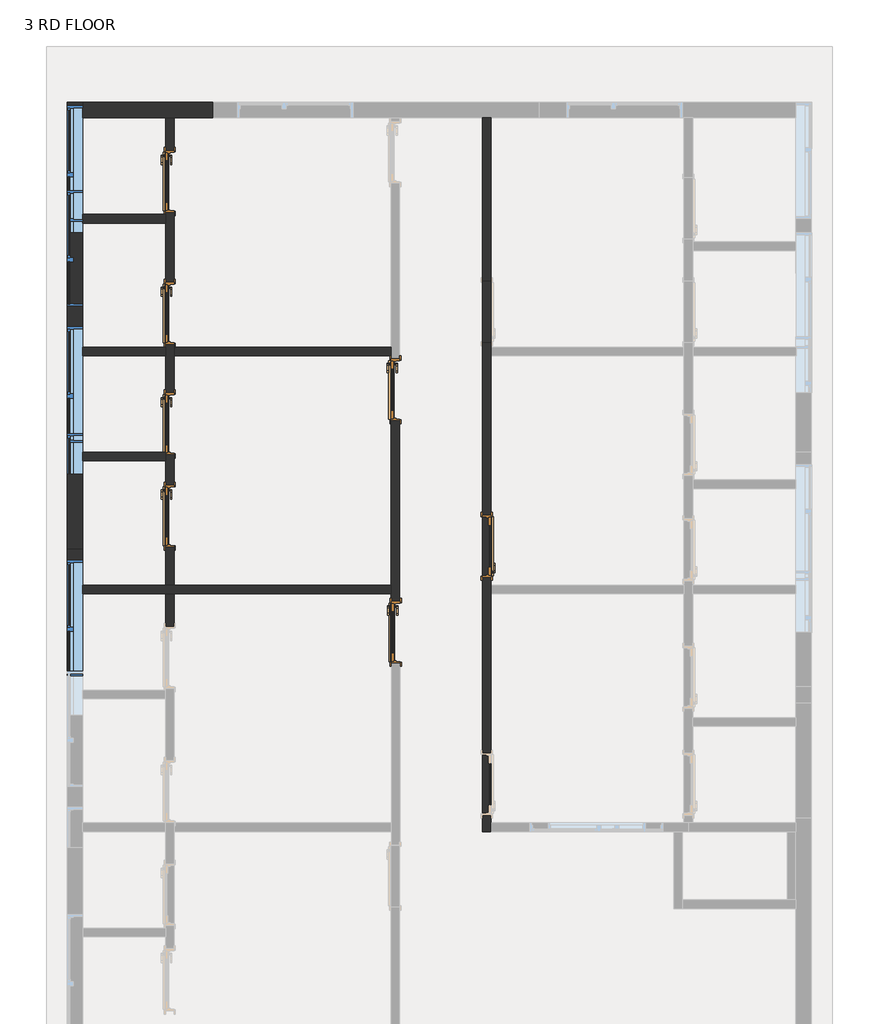
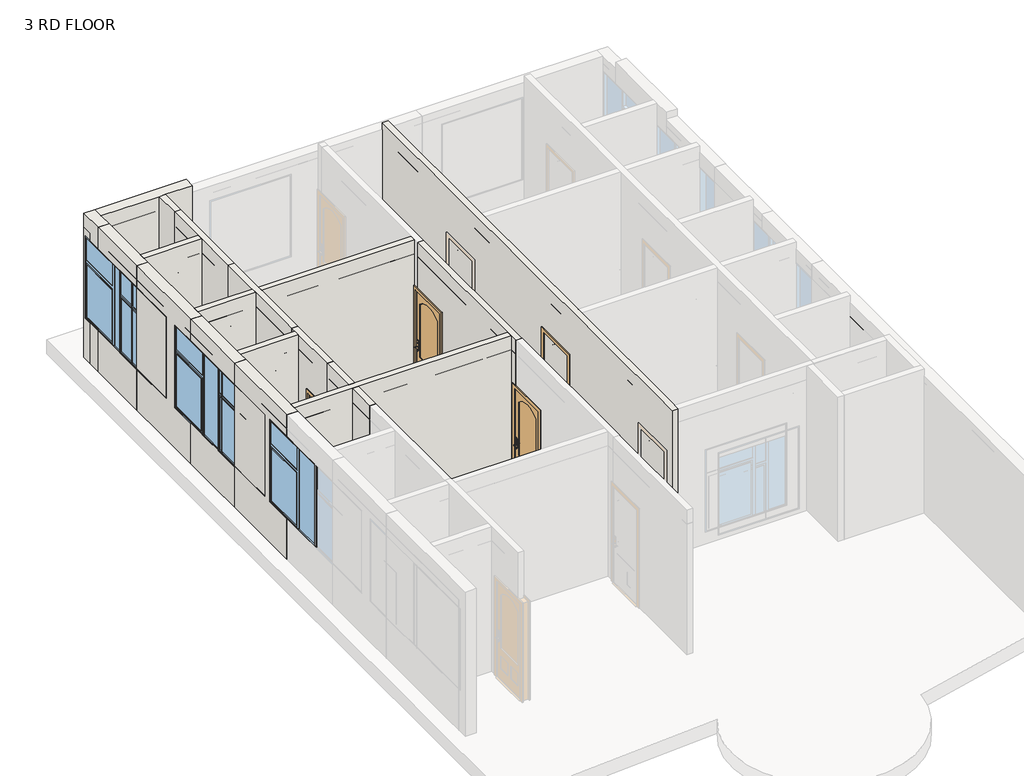
# One storey, part 2 of 5: 35 walls, 7 doors, 6 windows.
"""IFC4 building model written with IfcOpenShell, lengths in millimetres."""

from ifc_helpers import new_model, si_unit, frame, origin, place, context, project, spatial, polyline, outline, extrude, faceted_brep, transform, mapped, element, save
from components import door_346b4a94, m_window_casement_double_sidelight_1702_x_1829mm_c8b42c7f

model = new_model("IFC4")

# Units and contexts
model_context = context("Model", 3, world=origin())
ifc_project = project(units=[si_unit("LENGTHUNIT", "METRE", prefix="MILLI")], contexts=[model_context])

# Site, building, storey
site = spatial("IfcSite", under=ifc_project)
building = spatial("IfcBuilding", under=site)
storey = spatial("IfcBuildingStorey", under=building, Name="3 RD FLOOR", Elevation=9601.2)

# Doors
placement = place(None, origin())
door_shape = door_346b4a94(model_context)
element("IfcDoor", 1, ObjectType="2'10\"X7'", at=placement, inside=storey, context=model_context, shape_type="MappedRepresentation", body=[
    mapped(door_shape, transform((-273.0358866, 1471.0399728, 9601.2), x_axis=(0.0, -1.0, 0.0), y_axis=(1.0, 0.0, 0.0), z_axis=(0.0, 0.0, 1.0))),
])
element("IfcDoor", 2, ObjectType="2'10\"X7'", at=placement, inside=storey, context=model_context, shape_type="MappedRepresentation", body=[
    mapped(door_shape, transform((-4952.9858866, 3273.6174518, 9601.2), x_axis=(0.0, 1.0, 0.0), y_axis=(-1.0, 0.0, 0.0), z_axis=(0.0, 0.0, 1.0))),
])
element("IfcDoor", 3, ObjectType="2'10\"X7'", at=placement, inside=storey, context=model_context, shape_type="MappedRepresentation", body=[
    mapped(door_shape, transform((-4952.9858866, 4900.320652, 9601.2), x_axis=(0.0, 1.0, 0.0), y_axis=(-1.0, 0.0, 0.0), z_axis=(0.0, 0.0, 1.0))),
])
element("IfcDoor", 4, ObjectType="2'10\"X7'", at=placement, inside=storey, context=model_context, shape_type="MappedRepresentation", body=[
    mapped(door_shape, transform((-4952.9858866, 6843.9929737, 9601.2), x_axis=(0.0, 1.0, 0.0), y_axis=(-1.0, 0.0, 0.0), z_axis=(0.0, 0.0, 1.0))),
])
element("IfcDoor", 5, ObjectType="2'10\"X7'", at=placement, inside=storey, context=model_context, shape_type="MappedRepresentation", body=[
    mapped(door_shape, transform((-1625.1621817, 3775.8008884, 9601.2), x_axis=(0.0, 1.0, 0.0), y_axis=(-1.0, 0.0, 0.0), z_axis=(0.0, 0.0, 1.0))),
])
element("IfcDoor", 6, ObjectType="2'10\"X7'", at=placement, inside=storey, context=model_context, shape_type="MappedRepresentation", body=[
    mapped(door_shape, transform((-1620.1577262, 202.9637706, 9601.2), x_axis=(0.0, 1.0, 0.0), y_axis=(-1.0, 0.0, 0.0), z_axis=(0.0, 0.0, 1.0))),
])
element("IfcDoor", 7, ObjectType="2'10\"X7'", at=placement, inside=storey, context=model_context, shape_type="MappedRepresentation", body=[
    mapped(door_shape, transform((-4952.9858866, 1913.3521609, 9601.2), x_axis=(0.0, 1.0, 0.0), y_axis=(-1.0, 0.0, 0.0), z_axis=(0.0, 0.0, 1.0))),
])

# Walls
element("IfcWall", 8, ObjectType="Generic - 4.5\"", at=placement, inside=storey, context=model_context, shape_type="Brep", body=[
    faceted_brep([(-5013.3108866, 7224.9929737, 12801.6), (-5013.3108866, 7782.9399728, 12801.6), (-5013.3108866, 7782.9399728, 9601.2), (-5013.3108866, 7300.7929737, 9601.2), (-5013.3108866, 7300.7929737, 11759.8), (-5013.3108866, 7224.9929737, 11759.8), (-5013.3108866, 7224.9929737, 12496.8), (-4886.3108866, 7782.9399728, 12801.6), (-4886.3108866, 7224.9929737, 12801.6), (-4886.3108866, 7224.9929737, 12496.8), (-4886.3108866, 7224.9929737, 11759.8), (-4886.3108866, 7300.7929737, 11759.8), (-4886.3108866, 7300.7929737, 9601.2), (-4886.3108866, 7782.9399728, 9601.2)], [[[0, 1, 2, 3, 4, 5, 6]], [[7, 8, 9, 10, 11, 12, 13]], [[2, 13, 12, 3]], [[1, 0, 8, 7]], [[11, 4, 3, 12]], [[4, 11, 10, 5]], [[8, 0, 6, 5, 10, 9]], [[1, 7, 13, 2]]]),
])
element("IfcWall", 9, ObjectType="Generic - 4.5\"", at=placement, inside=storey, context=model_context, shape_type="Brep", body=[
    faceted_brep([(-5013.3108866, 5281.320652, 12801.6), (-5013.3108866, 6233.5399728, 12801.6), (-5013.3108866, 6360.5399728, 12801.6), (-5013.3108866, 7224.9929737, 12801.6), (-5013.3108866, 7224.9929737, 12496.8), (-5013.3108866, 7224.9929737, 11759.8), (-5013.3108866, 6387.1929737, 11759.8), (-5013.3108866, 6387.1929737, 9601.2), (-5013.3108866, 6360.5399728, 9601.2), (-5013.3108866, 6233.5399728, 9601.2), (-5013.3108866, 5357.120652, 9601.2), (-5013.3108866, 5357.120652, 11759.8), (-5013.3108866, 5281.320652, 11759.8), (-5013.3108866, 5281.320652, 12496.8), (-4886.3108866, 7224.9929737, 12801.6), (-4886.3108866, 5281.320652, 12801.6), (-4886.3108866, 5281.320652, 12496.8), (-4886.3108866, 5281.320652, 11759.8), (-4886.3108866, 5357.120652, 11759.8), (-4886.3108866, 5357.120652, 9601.2), (-4886.3108866, 6387.1929737, 9601.2), (-4886.3108866, 6387.1929737, 11759.8), (-4886.3108866, 7224.9929737, 11759.8), (-4886.3108866, 7224.9929737, 12496.8)], [[[0, 1, 2, 3, 4, 5, 6, 7, 8, 9, 10, 11, 12, 13]], [[14, 15, 16, 17, 18, 19, 20, 21, 22, 23]], [[19, 10, 9, 8, 7, 20]], [[3, 2, 1, 0, 15, 14]], [[18, 11, 10, 19]], [[11, 18, 17, 12]], [[21, 6, 5, 22]], [[6, 21, 20, 7]], [[15, 0, 13, 12, 17, 16]], [[3, 14, 23, 22, 5, 4]]]),
])
element("IfcWall", 10, ObjectType="Generic - 4.5\"", at=placement, inside=storey, context=model_context, shape_type="SweptSolid", body=[
    extrude(outline(polyline([(-5013.3108866, 6233.5399728), (-6232.5508078, 6233.5399728), (-6232.5508078, 6360.5399728), (-5013.3108866, 6360.5399728), (-5013.3108866, 6233.5399728)])), frame((0.0, 0.0, 9601.2), z_axis=(0.0, 0.0, 1.0), x_axis=(1.0, 0.0, 0.0)), (0.0, 0.0, 1.0), 3200.4),
])
element("IfcWall", 11, ObjectType="Generic - 4.5\"", at=placement, inside=storey, context=model_context, shape_type="SweptSolid", body=[
    extrude(outline(polyline([(-5013.3108866, 4277.7399728), (-6232.5508078, 4277.7399728), (-6232.5508078, 4404.7399728), (-5013.3108866, 4404.7399728), (-5013.3108866, 4277.7399728)])), frame((0.0, 0.0, 9601.2), z_axis=(0.0, 0.0, 1.0), x_axis=(1.0, 0.0, 0.0)), (0.0, 0.0, 1.0), 3200.4),
])
element("IfcWall", 12, ObjectType="Generic - 4.5\"", at=placement, inside=storey, context=model_context, shape_type="Brep", body=[
    faceted_brep([(-5013.3108866, 2968.8174518, 12801.6), (-5013.3108866, 4277.7399728, 12801.6), (-5013.3108866, 4404.7399728, 12801.6), (-5013.3108866, 5281.320652, 12801.6), (-5013.3108866, 5281.320652, 12496.8), (-5013.3108866, 5281.320652, 11759.8), (-5013.3108866, 4443.520652, 11759.8), (-5013.3108866, 4443.520652, 9601.2), (-5013.3108866, 4404.7399728, 9601.2), (-5013.3108866, 4277.7399728, 9601.2), (-5013.3108866, 3730.4174518, 9601.2), (-5013.3108866, 3730.4174518, 11759.8), (-5013.3108866, 2968.8174518, 11759.8), (-5013.3108866, 2968.8174518, 12496.8), (-4886.3108866, 5281.320652, 12801.6), (-4886.3108866, 4404.7399728, 12801.6), (-4886.3108866, 4277.7399728, 12801.6), (-4886.3108866, 2968.8174518, 12801.6), (-4886.3108866, 2968.8174518, 12496.8), (-4886.3108866, 2968.8174518, 11759.8), (-4886.3108866, 3730.4174518, 11759.8), (-4886.3108866, 3730.4174518, 9601.2), (-4886.3108866, 4277.7399728, 9601.2), (-4886.3108866, 4404.7399728, 9601.2), (-4886.3108866, 4443.520652, 9601.2), (-4886.3108866, 4443.520652, 11759.8), (-4886.3108866, 5281.320652, 11759.8), (-4886.3108866, 5281.320652, 12496.8)], [[[0, 1, 2, 3, 4, 5, 6, 7, 8, 9, 10, 11, 12, 13]], [[14, 15, 16, 17, 18, 19, 20, 21, 22, 23, 24, 25, 26, 27]], [[21, 10, 9, 8, 7, 24, 23, 22]], [[3, 2, 1, 0, 17, 16, 15, 14]], [[20, 11, 10, 21]], [[11, 20, 19, 12]], [[25, 6, 5, 26]], [[6, 25, 24, 7]], [[3, 14, 27, 26, 5, 4]], [[17, 0, 13, 12, 19, 18]]]),
])
element("IfcWall", 13, ObjectType="Generic - 4.5\"", at=placement, inside=storey, context=model_context, shape_type="Brep", body=[
    faceted_brep([(-6232.5508078, 2728.3399728, 9601.2), (-5013.3108866, 2728.3399728, 9601.2), (-5013.3108866, 2728.3399728, 12801.6), (-6232.5508078, 2728.3399728, 12801.6), (-6232.5508078, 2855.3399728, 9601.2), (-6232.5508078, 2855.3399728, 12801.6), (-5013.3108866, 2855.3399728, 12801.6), (-5013.3108866, 2855.3399728, 9601.2), (-5013.3108866, 2816.8174518, 9601.2)], [[[0, 1, 2, 3]], [[4, 5, 6, 7]], [[1, 0, 4, 7, 8]], [[3, 2, 6, 5]], [[0, 3, 5, 4]], [[2, 1, 8, 7, 6]]]),
])
element("IfcWall", 14, ObjectType="Generic - 4.5\"", at=placement, inside=storey, context=model_context, shape_type="Brep", body=[
    faceted_brep([(-5013.3108866, 1684.7521609, 12801.6), (-5013.3108866, 2728.3399728, 12801.6), (-5013.3108866, 2855.3399728, 12801.6), (-5013.3108866, 2968.8174518, 12801.6), (-5013.3108866, 2968.8174518, 12496.8), (-5013.3108866, 2968.8174518, 11759.8), (-5013.3108866, 2816.8174518, 11759.8), (-5013.3108866, 2816.8174518, 9601.2), (-5013.3108866, 2728.3399728, 9601.2), (-5013.3108866, 2370.1521609, 9601.2), (-5013.3108866, 2370.1521609, 11759.8), (-5013.3108866, 1684.7521609, 11759.8), (-5013.3108866, 1684.7521609, 12496.8), (-4886.3108866, 2968.8174518, 12801.6), (-4886.3108866, 1684.7521609, 12801.6), (-4886.3108866, 1684.7521609, 12496.8), (-4886.3108866, 1684.7521609, 11759.8), (-4886.3108866, 2370.1521609, 11759.8), (-4886.3108866, 2370.1521609, 9601.2), (-4886.3108866, 2816.8174518, 9601.2), (-4886.3108866, 2816.8174518, 11759.8), (-4886.3108866, 2968.8174518, 11759.8), (-4886.3108866, 2968.8174518, 12496.8)], [[[0, 1, 2, 3, 4, 5, 6, 7, 8, 9, 10, 11, 12]], [[13, 14, 15, 16, 17, 18, 19, 20, 21, 22]], [[7, 19, 18, 9, 8]], [[3, 2, 1, 0, 14, 13]], [[20, 6, 5, 21]], [[6, 20, 19, 7]], [[17, 10, 9, 18]], [[10, 17, 16, 11]], [[3, 13, 22, 21, 5, 4]], [[14, 0, 12, 11, 16, 15]]]),
])
element("IfcWall", 15, ObjectType="Generic - 4.5\"", at=placement, inside=storey, context=model_context, shape_type="Brep", body=[
    faceted_brep([(-6232.5508078, 772.5399728, 9601.2), (-5013.3108866, 772.5399728, 9601.2), (-4886.3108866, 772.5399728, 9601.2), (-1685.9108866, 772.5399728, 9601.2), (-1685.9108866, 772.5399728, 12801.6), (-4886.3108866, 772.5399728, 12801.6), (-5013.3108866, 772.5399728, 12801.6), (-6232.5508078, 772.5399728, 12801.6), (-6232.5508078, 899.5399728, 9601.2), (-6232.5508078, 899.5399728, 12801.6), (-5013.3108866, 899.5399728, 12801.6), (-4886.3108866, 899.5399728, 12801.6), (-1685.9108866, 899.5399728, 12801.6), (-1685.9108866, 899.5399728, 9601.2), (-4886.3108866, 899.5399728, 9601.2), (-5013.3108866, 899.5399728, 9601.2)], [[[0, 1, 2, 3, 4, 5, 6, 7]], [[8, 9, 10, 11, 12, 13, 14, 15]], [[3, 2, 1, 0, 8, 15, 14, 13]], [[4, 3, 13, 12]], [[7, 6, 5, 4, 12, 11, 10, 9]], [[0, 7, 9, 8]]]),
])
element("IfcWall", 16, ObjectType="Generic - 4.5\"", at=placement, inside=storey, context=model_context, shape_type="Brep", body=[
    faceted_brep([(-5013.3108866, 288.8295043, 9601.2), (-5013.3108866, 288.8295043, 11759.8), (-5013.3108866, 136.8295043, 11759.8), (-5013.3108866, 136.8295043, 12496.8), (-5013.3108866, 136.8295043, 12801.6), (-5013.3108866, 772.5399728, 12801.6), (-5013.3108866, 772.5399728, 9601.2), (-4886.3108866, 288.8295043, 11759.8), (-4886.3108866, 288.8295043, 9601.2), (-4886.3108866, 772.5399728, 9601.2), (-4886.3108866, 772.5399728, 12801.6), (-4886.3108866, 136.8295043, 12801.6), (-4886.3108866, 136.8295043, 12496.8), (-4886.3108866, 136.8295043, 11759.8)], [[[0, 1, 2, 3, 4, 5, 6]], [[7, 8, 9, 10, 11, 12, 13]], [[8, 0, 6, 9]], [[4, 11, 10, 5]], [[7, 1, 0, 8]], [[1, 7, 13, 2]], [[6, 5, 10, 9]], [[11, 4, 3, 2, 13, 12]]]),
    faceted_brep([(-5013.3108866, 1684.7521609, 11759.8), (-5013.3108866, 1456.5521609, 11759.8), (-5013.3108866, 1456.5521609, 9601.2), (-5013.3108866, 899.5399728, 9601.2), (-5013.3108866, 899.5399728, 12801.6), (-5013.3108866, 1684.7521609, 12801.6), (-5013.3108866, 1684.7521609, 12496.8), (-4886.3108866, 1456.5521609, 11759.8), (-4886.3108866, 1684.7521609, 11759.8), (-4886.3108866, 1684.7521609, 12496.8), (-4886.3108866, 1684.7521609, 12801.6), (-4886.3108866, 899.5399728, 12801.6), (-4886.3108866, 899.5399728, 9601.2), (-4886.3108866, 1456.5521609, 9601.2)], [[[0, 1, 2, 3, 4, 5, 6]], [[7, 8, 9, 10, 11, 12, 13]], [[2, 13, 12, 3]], [[10, 5, 4, 11]], [[4, 3, 12, 11]], [[7, 1, 0, 8]], [[1, 7, 13, 2]], [[5, 10, 9, 8, 0, 6]]]),
])
element("IfcWall", 17, ObjectType="Generic - 4.5\"", at=placement, inside=storey, context=model_context, shape_type="SweptSolid", body=[
    extrude(outline(polyline([(-1685.9108866, 4277.7399728), (-4886.3108866, 4277.7399728), (-4886.3108866, 4404.7399728), (-1685.9108866, 4404.7399728), (-1685.9108866, 4277.7399728)])), frame((0.0, 0.0, 9601.2), z_axis=(0.0, 0.0, 1.0), x_axis=(1.0, 0.0, 0.0)), (0.0, 0.0, 1.0), 3200.4),
])
element("IfcWall", 18, ObjectType="Generic - 4.5\"", at=placement, inside=storey, context=model_context, shape_type="Brep", body=[
    faceted_brep([(-1685.4871817, 609.3637706, 12801.6), (-1685.4871817, 4182.2008884, 12801.6), (-1685.4871817, 4182.2008884, 11759.8), (-1685.4871817, 3319.0008884, 11759.8), (-1685.4871817, 3319.0008884, 9601.2), (-1685.4871817, 659.7637706, 9601.2), (-1685.4871817, 659.7637706, 11759.8), (-1685.4871817, 609.3637706, 11759.8), (-1558.4871817, 4182.2008884, 12801.6), (-1558.4871817, 609.3637706, 12801.6), (-1558.4871817, 609.3637706, 11759.8), (-1558.4871817, 659.7637706, 11759.8), (-1558.4871817, 659.7637706, 9601.2), (-1558.4871817, 3319.0008884, 9601.2), (-1558.4871817, 3319.0008884, 11759.8), (-1558.4871817, 4182.2008884, 11759.8), (-1680.4827262, 609.3637706, 12801.6), (-1558.9108866, 4182.2008884, 12801.6), (-1558.9108866, 4182.2008884, 11759.8), (-1680.4827262, 609.3637706, 11759.8)], [[[0, 1, 2, 3, 4, 5, 6, 7]], [[8, 9, 10, 11, 12, 13, 14, 15]], [[4, 13, 12, 5]], [[1, 0, 16, 9, 8, 17]], [[14, 3, 2, 18, 15]], [[3, 14, 13, 4]], [[11, 6, 5, 12]], [[6, 11, 10, 19, 7]], [[9, 16, 0, 7, 19, 10]], [[1, 17, 8, 15, 18, 2]]]),
])
element("IfcWall", 19, ObjectType="Generic - 4.5\"", at=placement, inside=storey, context=model_context, shape_type="Brep", body=[
    faceted_brep([(-339.7108866, -2732.6600272, 12801.6), (-339.7108866, 7782.9399728, 12801.6), (-339.7108866, 7782.9399728, 9601.2), (-339.7108866, 5382.2399728, 9601.2), (-339.7108866, 5382.2399728, 11759.8), (-339.7108866, 4468.6399728, 11759.8), (-339.7108866, 4468.6399728, 9601.2), (-339.7108866, 1927.8399728, 9601.2), (-339.7108866, 1927.8399728, 11759.8), (-339.7108866, 1014.2399728, 11759.8), (-339.7108866, 1014.2399728, 9601.2), (-339.7108866, -1577.3600272, 9601.2), (-339.7108866, -1577.3600272, 11759.8), (-339.7108866, -2490.9600272, 11759.8), (-339.7108866, -2490.9600272, 9601.2), (-339.7108866, -2732.6600272, 9601.2), (-212.7108866, 7782.9399728, 12801.6), (-212.7108866, 4404.7399728, 12801.6), (-212.7108866, 4277.7399728, 12801.6), (-212.7108866, 899.5399728, 12801.6), (-212.7108866, 772.5399728, 12801.6), (-212.7108866, -2605.6600272, 12801.6), (-212.7108866, -2732.6600272, 12801.6), (-212.7108866, -2732.6600272, 12496.8), (-212.7108866, -2732.6600272, 9601.2), (-212.7108866, -2605.6600272, 9601.2), (-212.7108866, -2490.9600272, 9601.2), (-212.7108866, -2490.9600272, 11759.8), (-212.7108866, -1577.3600272, 11759.8), (-212.7108866, -1577.3600272, 9601.2), (-212.7108866, 772.5399728, 9601.2), (-212.7108866, 899.5399728, 9601.2), (-212.7108866, 1014.2399728, 9601.2), (-212.7108866, 1014.2399728, 11759.8), (-212.7108866, 1927.8399728, 11759.8), (-212.7108866, 1927.8399728, 9601.2), (-212.7108866, 4277.7399728, 9601.2), (-212.7108866, 4404.7399728, 9601.2), (-212.7108866, 4468.6399728, 9601.2), (-212.7108866, 4468.6399728, 11759.8), (-212.7108866, 5382.2399728, 11759.8), (-212.7108866, 5382.2399728, 9601.2), (-212.7108866, 7782.9399728, 9601.2)], [[[0, 1, 2, 3, 4, 5, 6, 7, 8, 9, 10, 11, 12, 13, 14, 15]], [[16, 17, 18, 19, 20, 21, 22, 23, 24, 25, 26, 27, 28, 29, 30, 31, 32, 33, 34, 35, 36, 37, 38, 39, 40, 41, 42]], [[24, 15, 14, 26, 25]], [[29, 11, 10, 32, 31, 30]], [[35, 7, 6, 38, 37, 36]], [[2, 42, 41, 3]], [[1, 0, 22, 21, 20, 19, 18, 17, 16]], [[13, 27, 26, 14]], [[27, 13, 12, 28]], [[28, 12, 11, 29]], [[9, 33, 32, 10]], [[33, 9, 8, 34]], [[34, 8, 7, 35]], [[5, 39, 38, 6]], [[39, 5, 4, 40]], [[40, 4, 3, 41]], [[15, 24, 23, 22, 0]], [[1, 16, 42, 2]]]),
])
element("IfcWall", 20, ObjectType="Generic - 4.5\"", at=placement, inside=storey, context=model_context, shape_type="SweptSolid", body=[
    extrude(outline(polyline([(7782.9399728, 12496.8), (7782.9399728, 9601.2), (7300.7929737, 9601.2), (7300.7929737, 11759.8), (7224.9929737, 11759.8), (7224.9929737, 12496.8), (7782.9399728, 12496.8)])), frame((-5013.3108866, 0.0, 0.0), z_axis=(1.0, 0.0, 0.0), x_axis=(0.0, 1.0, 0.0)), (0.0, 0.0, 1.0), 127.0),
])
element("IfcWall", 21, ObjectType="Generic - 4.5\"", at=placement, inside=storey, context=model_context, shape_type="Brep", body=[
    faceted_brep([(-5013.3108866, 5281.320652, 12496.8), (-5013.3108866, 6233.5399728, 12496.8), (-5013.3108866, 6360.5399728, 12496.8), (-5013.3108866, 7224.9929737, 12496.8), (-5013.3108866, 7224.9929737, 11759.8), (-5013.3108866, 6387.1929737, 11759.8), (-5013.3108866, 6387.1929737, 9601.2), (-5013.3108866, 6360.5399728, 9601.2), (-5013.3108866, 6233.5399728, 9601.2), (-5013.3108866, 5357.120652, 9601.2), (-5013.3108866, 5357.120652, 11759.8), (-5013.3108866, 5281.320652, 11759.8), (-4886.3108866, 7224.9929737, 12496.8), (-4886.3108866, 5281.320652, 12496.8), (-4886.3108866, 5281.320652, 11759.8), (-4886.3108866, 5357.120652, 11759.8), (-4886.3108866, 5357.120652, 9601.2), (-4886.3108866, 6387.1929737, 9601.2), (-4886.3108866, 6387.1929737, 11759.8), (-4886.3108866, 7224.9929737, 11759.8)], [[[0, 1, 2, 3, 4, 5, 6, 7, 8, 9, 10, 11]], [[12, 13, 14, 15, 16, 17, 18, 19]], [[16, 9, 8, 7, 6, 17]], [[13, 0, 11, 14]], [[3, 12, 19, 4]], [[3, 2, 1, 0, 13, 12]], [[18, 5, 4, 19]], [[5, 18, 17, 6]], [[15, 10, 9, 16]], [[10, 15, 14, 11]]]),
])
element("IfcWall", 22, ObjectType="Generic - 4.5\"", at=placement, inside=storey, context=model_context, shape_type="SweptSolid", body=[
    extrude(outline(polyline([(-5013.3108866, 6233.5399728), (-6232.5508078, 6233.5399728), (-6232.5508078, 6360.5399728), (-5013.3108866, 6360.5399728), (-5013.3108866, 6233.5399728)])), frame((0.0, 0.0, 9601.2), z_axis=(0.0, 0.0, 1.0), x_axis=(1.0, 0.0, 0.0)), (0.0, 0.0, 1.0), 2895.6),
])
element("IfcWall", 23, ObjectType="Generic - 4.5\"", at=placement, inside=storey, context=model_context, shape_type="SweptSolid", body=[
    extrude(outline(polyline([(-5013.3108866, 4277.7399728), (-6232.5508078, 4277.7399728), (-6232.5508078, 4404.7399728), (-5013.3108866, 4404.7399728), (-5013.3108866, 4277.7399728)])), frame((0.0, 0.0, 9601.2), z_axis=(0.0, 0.0, 1.0), x_axis=(1.0, 0.0, 0.0)), (0.0, 0.0, 1.0), 2895.6),
])
element("IfcWall", 24, ObjectType="Generic - 4.5\"", at=placement, inside=storey, context=model_context, shape_type="Brep", body=[
    faceted_brep([(-5013.3108866, 2968.8174518, 12496.8), (-5013.3108866, 4277.7399728, 12496.8), (-5013.3108866, 4404.7399728, 12496.8), (-5013.3108866, 5281.320652, 12496.8), (-5013.3108866, 5281.320652, 11759.8), (-5013.3108866, 4443.520652, 11759.8), (-5013.3108866, 4443.520652, 9601.2), (-5013.3108866, 4404.7399728, 9601.2), (-5013.3108866, 4277.7399728, 9601.2), (-5013.3108866, 3730.4174518, 9601.2), (-5013.3108866, 3730.4174518, 11759.8), (-5013.3108866, 2968.8174518, 11759.8), (-4886.3108866, 5281.320652, 12496.8), (-4886.3108866, 4404.7399728, 12496.8), (-4886.3108866, 4277.7399728, 12496.8), (-4886.3108866, 2968.8174518, 12496.8), (-4886.3108866, 2968.8174518, 11759.8), (-4886.3108866, 3730.4174518, 11759.8), (-4886.3108866, 3730.4174518, 9601.2), (-4886.3108866, 4277.7399728, 9601.2), (-4886.3108866, 4404.7399728, 9601.2), (-4886.3108866, 4443.520652, 9601.2), (-4886.3108866, 4443.520652, 11759.8), (-4886.3108866, 5281.320652, 11759.8)], [[[0, 1, 2, 3, 4, 5, 6, 7, 8, 9, 10, 11]], [[12, 13, 14, 15, 16, 17, 18, 19, 20, 21, 22, 23]], [[18, 9, 8, 7, 6, 21, 20, 19]], [[15, 0, 11, 16]], [[3, 12, 23, 4]], [[3, 2, 1, 0, 15, 14, 13, 12]], [[22, 5, 4, 23]], [[5, 22, 21, 6]], [[17, 10, 9, 18]], [[10, 17, 16, 11]]]),
])
element("IfcWall", 25, ObjectType="Generic - 4.5\"", at=placement, inside=storey, context=model_context, shape_type="Brep", body=[
    faceted_brep([(-6232.5508078, 2728.3399728, 9601.2), (-5013.3108866, 2728.3399728, 9601.2), (-5013.3108866, 2728.3399728, 12496.8), (-6232.5508078, 2728.3399728, 12496.8), (-6232.5508078, 2855.3399728, 9601.2), (-6232.5508078, 2855.3399728, 12496.8), (-5013.3108866, 2855.3399728, 12496.8), (-5013.3108866, 2855.3399728, 9601.2), (-5013.3108866, 2816.8174518, 9601.2)], [[[0, 1, 2, 3]], [[4, 5, 6, 7]], [[1, 0, 4, 7, 8]], [[0, 3, 5, 4]], [[2, 1, 8, 7, 6]], [[3, 2, 6, 5]]]),
])
element("IfcWall", 26, ObjectType="Generic - 4.5\"", at=placement, inside=storey, context=model_context, shape_type="Brep", body=[
    faceted_brep([(-5013.3108866, 1684.7521609, 12496.8), (-5013.3108866, 2728.3399728, 12496.8), (-5013.3108866, 2855.3399728, 12496.8), (-5013.3108866, 2968.8174518, 12496.8), (-5013.3108866, 2968.8174518, 11759.8), (-5013.3108866, 2816.8174518, 11759.8), (-5013.3108866, 2816.8174518, 9601.2), (-5013.3108866, 2728.3399728, 9601.2), (-5013.3108866, 2370.1521609, 9601.2), (-5013.3108866, 2370.1521609, 11759.8), (-5013.3108866, 1684.7521609, 11759.8), (-4886.3108866, 2968.8174518, 12496.8), (-4886.3108866, 1684.7521609, 12496.8), (-4886.3108866, 1684.7521609, 11759.8), (-4886.3108866, 2370.1521609, 11759.8), (-4886.3108866, 2370.1521609, 9601.2), (-4886.3108866, 2816.8174518, 9601.2), (-4886.3108866, 2816.8174518, 11759.8), (-4886.3108866, 2968.8174518, 11759.8)], [[[0, 1, 2, 3, 4, 5, 6, 7, 8, 9, 10]], [[11, 12, 13, 14, 15, 16, 17, 18]], [[6, 16, 15, 8, 7]], [[12, 0, 10, 13]], [[3, 11, 18, 4]], [[3, 2, 1, 0, 12, 11]], [[14, 9, 8, 15]], [[9, 14, 13, 10]], [[17, 5, 4, 18]], [[5, 17, 16, 6]]]),
])
element("IfcWall", 27, ObjectType="Generic - 4.5\"", at=placement, inside=storey, context=model_context, shape_type="SweptSolid", body=[
    extrude(outline(polyline([(-1685.9108866, 899.5399728), (-1685.9108866, 772.5399728), (-4886.3108866, 772.5399728), (-4886.3108866, 899.5399728), (-1685.9108866, 899.5399728)])), frame((0.0, 0.0, 9601.2), z_axis=(0.0, 0.0, 1.0), x_axis=(1.0, 0.0, 0.0)), (0.0, 0.0, 1.0), 2895.6),
    extrude(outline(polyline([(-6232.5508078, 772.5399728), (-6232.5508078, 899.5399728), (-5013.3108866, 899.5399728), (-5013.3108866, 772.5399728), (-6232.5508078, 772.5399728)])), frame((0.0, 0.0, 9601.2), z_axis=(0.0, 0.0, 1.0), x_axis=(1.0, 0.0, 0.0)), (0.0, 0.0, 1.0), 2895.6),
])
element("IfcWall", 28, ObjectType="Generic - 4.5\"", at=placement, inside=storey, context=model_context, shape_type="SweptSolid", body=[
    extrude(outline(polyline([(772.5399728, 12496.8), (772.5399728, 9601.2), (288.8295043, 9601.2), (288.8295043, 11759.8), (136.8295043, 11759.8), (136.8295043, 12496.8), (772.5399728, 12496.8)])), frame((-5013.3108866, 0.0, 0.0), z_axis=(1.0, 0.0, 0.0), x_axis=(0.0, 1.0, 0.0)), (0.0, 0.0, 1.0), 127.0),
    extrude(outline(polyline([(899.5399728, 9601.2), (899.5399728, 12496.8), (1684.7521609, 12496.8), (1684.7521609, 11759.8), (1456.5521609, 11759.8), (1456.5521609, 9601.2), (899.5399728, 9601.2)])), frame((-5013.3108866, 0.0, 0.0), z_axis=(1.0, 0.0, 0.0), x_axis=(0.0, 1.0, 0.0)), (0.0, 0.0, 1.0), 127.0),
])
element("IfcWall", 29, ObjectType="Generic - 4.5\"", at=placement, inside=storey, context=model_context, shape_type="Brep", body=[
    faceted_brep([(-1685.4871817, 609.3637706, 12496.8), (-1685.4871817, 4182.2008884, 12496.8), (-1685.4871817, 4182.2008884, 11759.8), (-1685.4871817, 3319.0008884, 11759.8), (-1685.4871817, 3319.0008884, 9601.2), (-1685.4871817, 659.7637706, 9601.2), (-1685.4871817, 659.7637706, 11759.8), (-1685.4871817, 609.3637706, 11759.8), (-1558.4871817, 4182.2008884, 12496.8), (-1558.4871817, 609.3637706, 12496.8), (-1558.4871817, 609.3637706, 11759.8), (-1558.4871817, 659.7637706, 11759.8), (-1558.4871817, 659.7637706, 9601.2), (-1558.4871817, 3319.0008884, 9601.2), (-1558.4871817, 3319.0008884, 11759.8), (-1558.4871817, 4182.2008884, 11759.8), (-1680.4827262, 609.3637706, 12496.8), (-1680.4827262, 609.3637706, 11759.8), (-1558.9108866, 4182.2008884, 12496.8), (-1558.9108866, 4182.2008884, 11759.8)], [[[0, 1, 2, 3, 4, 5, 6, 7]], [[8, 9, 10, 11, 12, 13, 14, 15]], [[4, 13, 12, 5]], [[9, 16, 0, 7, 17, 10]], [[1, 18, 8, 15, 19, 2]], [[1, 0, 16, 9, 8, 18]], [[11, 6, 5, 12]], [[6, 11, 10, 17, 7]], [[14, 3, 2, 19, 15]], [[3, 14, 13, 4]]]),
])
element("IfcWall", 30, ObjectType="Generic - 4.5\"", at=placement, inside=storey, context=model_context, shape_type="Brep", body=[
    faceted_brep([(-339.7108866, 7782.9399728, 9601.2), (-339.7108866, -2605.6600272, 9601.2), (-339.7108866, -2605.6600272, 12496.8), (-339.7108866, 7782.9399728, 12496.8), (-212.7108866, 7782.9399728, 9601.2), (-212.7108866, 7782.9399728, 12496.8), (-212.7108866, 4404.7399728, 12496.8), (-212.7108866, 4277.7399728, 12496.8), (-212.7108866, 899.5399728, 12496.8), (-212.7108866, 772.5399728, 12496.8), (-212.7108866, -2605.6600272, 12496.8), (-212.7108866, -2605.6600272, 9601.2), (-212.7108866, 772.5399728, 9601.2), (-212.7108866, 899.5399728, 9601.2), (-212.7108866, 4277.7399728, 9601.2), (-212.7108866, 4404.7399728, 9601.2)], [[[0, 1, 2, 3]], [[4, 5, 6, 7, 8, 9, 10, 11, 12, 13, 14, 15]], [[1, 0, 4, 15, 14, 13, 12, 11]], [[0, 3, 5, 4]], [[3, 2, 10, 9, 8, 7, 6, 5]], [[2, 1, 11, 10]]]),
])
element("IfcWall", 31, ObjectType="Generic - 9\"", at=placement, inside=storey, context=model_context, shape_type="Brep", body=[
    faceted_brep([(-6232.5108866, 7782.9399728, 12801.6), (-6232.5108866, 7782.9399728, 9601.2), (-5013.3108866, 7782.9399728, 9601.2), (-4886.3108866, 7782.9399728, 9601.2), (-4318.2603585, 7782.9399728, 9601.2), (-4318.2603585, 7782.9399728, 12496.8), (-4318.2603585, 7782.9399728, 12649.2), (-4318.2603585, 7782.9399728, 12801.6), (-4886.3108866, 7782.9399728, 12801.6), (-5013.3108866, 7782.9399728, 12801.6), (-6232.5108866, 8011.5399728, 9601.2), (-6232.5108866, 8011.5399728, 12496.8), (-6232.5108866, 8011.5399728, 12801.6), (-4318.2603585, 8011.5399728, 12801.6), (-4318.2603585, 8011.5399728, 12649.2), (-4318.2603585, 8011.5399728, 12496.8), (-4318.2603585, 8011.5399728, 9601.2)], [[[0, 1, 2, 3, 4, 5, 6, 7, 8, 9]], [[10, 11, 12, 13, 14, 15, 16]], [[4, 3, 2, 1, 10, 16]], [[0, 9, 8, 7, 13, 12]], [[4, 16, 15, 14, 13, 7, 6, 5]], [[0, 12, 11, 10, 1]]]),
])
element("IfcWall", 32, ObjectType="Generic - 9\"", at=placement, inside=storey, context=model_context, shape_type="Brep", body=[
    faceted_brep([(-6232.5508078, 642.0011338, 9601.2), (-6232.5508078, 772.5399728, 9601.2), (-6232.5508078, 899.5399728, 9601.2), (-6232.5508078, 2534.5107865, 9601.2), (-6232.5508078, 2534.5107865, 10501.2), (-6232.5508078, 1429.6107865, 10501.2), (-6232.5508078, 1429.6107865, 12330.0), (-6232.5508078, 2534.5107865, 12330.0), (-6232.5508078, 2534.5107865, 12496.8), (-6232.5508078, 2534.5107865, 12801.6), (-6232.5508078, 899.5399728, 12801.6), (-6232.5508078, 772.5399728, 12801.6), (-6232.5508078, 642.0011338, 12801.6), (-6232.5508078, 642.0011338, 12496.8), (-6232.5508078, 642.0011338, 12330.0), (-6232.5508078, 1264.3011338, 12330.0), (-6232.5508078, 1264.3011338, 10501.2), (-6232.5508078, 642.0011338, 10501.2), (-6461.1508078, 2534.5107865, 9601.2), (-6461.1508078, 642.0011338, 9601.2), (-6461.1508078, 642.0011338, 10501.2), (-6461.1508078, 1264.3011338, 10501.2), (-6461.1508078, 1264.3011338, 12330.0), (-6461.1508078, 642.0011338, 12330.0), (-6461.1508078, 642.0011338, 12496.8), (-6461.1508078, 642.0011338, 12801.6), (-6461.1508078, 2534.5107865, 12801.6), (-6461.1508078, 2534.5107865, 12496.8), (-6461.1508078, 2534.5107865, 12330.0), (-6461.1508078, 1429.6107865, 12330.0), (-6461.1508078, 1429.6107865, 10501.2), (-6461.1508078, 2534.5107865, 10501.2)], [[[0, 1, 2, 3, 4, 5, 6, 7, 8, 9, 10, 11, 12, 13, 14, 15, 16, 17]], [[18, 19, 20, 21, 22, 23, 24, 25, 26, 27, 28, 29, 30, 31]], [[3, 2, 1, 0, 19, 18]], [[12, 11, 10, 9, 26, 25]], [[30, 5, 4, 31]], [[5, 30, 29, 6]], [[6, 29, 28, 7]], [[15, 22, 21, 16]], [[16, 21, 20, 17]], [[22, 15, 14, 23]], [[12, 25, 24, 23, 14, 13]], [[19, 0, 17, 20]], [[26, 9, 8, 7, 28, 27]], [[3, 18, 31, 4]]]),
])
element("IfcWall", 33, ObjectType="Generic - 9\"", at=placement, inside=storey, context=model_context, shape_type="Brep", body=[
    faceted_brep([(-6232.5508078, 2534.5107865, 9601.2), (-6232.5508078, 2728.3399728, 9601.2), (-6232.5508078, 2855.3399728, 9601.2), (-6232.5508078, 4130.2388609, 9601.2), (-6232.5508078, 4130.2388609, 10501.2), (-6232.5508078, 2534.5107865, 10501.2), (-6461.1508078, 4130.2388609, 9601.2), (-6461.1508078, 2534.5107865, 9601.2), (-6461.1508078, 2534.5107865, 10501.2), (-6461.1508078, 4130.2388609, 10501.2)], [[[0, 1, 2, 3, 4, 5]], [[6, 7, 8, 9]], [[3, 2, 1, 0, 7, 6]], [[4, 9, 8, 5]], [[7, 0, 5, 8]], [[3, 6, 9, 4]]]),
    faceted_brep([(-6232.5508078, 4130.2388609, 12801.6), (-6232.5508078, 2855.3399728, 12801.6), (-6232.5508078, 2728.3399728, 12801.6), (-6232.5508078, 2534.5107865, 12801.6), (-6232.5508078, 2534.5107865, 12496.8), (-6232.5508078, 2534.5107865, 12330.0), (-6232.5508078, 4130.2388609, 12330.0), (-6232.5508078, 4130.2388609, 12496.8), (-6461.1508078, 2534.5107865, 12801.6), (-6461.1508078, 4130.2388609, 12801.6), (-6461.1508078, 4130.2388609, 12496.8), (-6461.1508078, 4130.2388609, 12330.0), (-6461.1508078, 2534.5107865, 12330.0), (-6461.1508078, 2534.5107865, 12496.8)], [[[0, 1, 2, 3, 4, 5, 6, 7]], [[8, 9, 10, 11, 12, 13]], [[3, 2, 1, 0, 9, 8]], [[11, 6, 5, 12]], [[3, 8, 13, 12, 5, 4]], [[9, 0, 7, 6, 11, 10]]]),
])
element("IfcWall", 34, ObjectType="Generic - 9\"", at=placement, inside=storey, context=model_context, shape_type="Brep", body=[
    faceted_brep([(-6232.5508078, 4130.2388609, 9601.2), (-6232.5508078, 4277.7399728, 9601.2), (-6232.5508078, 4404.7399728, 9601.2), (-6232.5508078, 6088.0863192, 9601.2), (-6232.5508078, 6088.0863192, 10501.2), (-6232.5508078, 5008.5863192, 10501.2), (-6232.5508078, 5008.5863192, 12330.0), (-6232.5508078, 6088.0863192, 12330.0), (-6232.5508078, 6088.0863192, 12496.8), (-6232.5508078, 6088.0863192, 12801.6), (-6232.5508078, 4404.7399728, 12801.6), (-6232.5508078, 4277.7399728, 12801.6), (-6232.5508078, 4130.2388609, 12801.6), (-6232.5508078, 4130.2388609, 12496.8), (-6232.5508078, 4130.2388609, 12330.0), (-6232.5508078, 4701.7388609, 12330.0), (-6232.5508078, 4701.7388609, 10501.2), (-6232.5508078, 4130.2388609, 10501.2), (-6461.1508078, 6088.0863192, 9601.2), (-6461.1508078, 4130.2388609, 9601.2), (-6461.1508078, 4130.2388609, 10501.2), (-6461.1508078, 4701.7388609, 10501.2), (-6461.1508078, 4701.7388609, 12330.0), (-6461.1508078, 4130.2388609, 12330.0), (-6461.1508078, 4130.2388609, 12496.8), (-6461.1508078, 4130.2388609, 12801.6), (-6461.1508078, 6088.0863192, 12801.6), (-6461.1508078, 6088.0863192, 12496.8), (-6461.1508078, 6088.0863192, 12330.0), (-6461.1508078, 5008.5863192, 12330.0), (-6461.1508078, 5008.5863192, 10501.2), (-6461.1508078, 6088.0863192, 10501.2)], [[[0, 1, 2, 3, 4, 5, 6, 7, 8, 9, 10, 11, 12, 13, 14, 15, 16, 17]], [[18, 19, 20, 21, 22, 23, 24, 25, 26, 27, 28, 29, 30, 31]], [[3, 2, 1, 0, 19, 18]], [[12, 11, 10, 9, 26, 25]], [[30, 5, 4, 31]], [[5, 30, 29, 6]], [[6, 29, 28, 7]], [[15, 22, 21, 16]], [[16, 21, 20, 17]], [[22, 15, 14, 23]], [[12, 25, 24, 23, 14, 13]], [[19, 0, 17, 20]], [[26, 9, 8, 7, 28, 27]], [[3, 18, 31, 4]]]),
])
element("IfcWall", 35, ObjectType="Generic - 9\"", at=placement, inside=storey, context=model_context, shape_type="Brep", body=[
    faceted_brep([(-6232.5508078, 6088.0863192, 9601.2), (-6232.5508078, 6233.5399728, 9601.2), (-6232.5508078, 6360.5399728, 9601.2), (-6232.5508078, 7490.3748838, 9601.2), (-6232.5508078, 7490.3748838, 10501.2), (-6232.5508078, 6088.0863192, 10501.2), (-6461.1508078, 7490.3748838, 9601.2), (-6461.1508078, 6088.0863192, 9601.2), (-6461.1508078, 6088.0863192, 10501.2), (-6461.1508078, 7490.3748838, 10501.2)], [[[0, 1, 2, 3, 4, 5]], [[6, 7, 8, 9]], [[3, 2, 1, 0, 7, 6]], [[4, 9, 8, 5]], [[7, 0, 5, 8]], [[3, 6, 9, 4]]]),
    faceted_brep([(-6232.5508078, 7490.3748838, 12801.6), (-6232.5508078, 6360.5399728, 12801.6), (-6232.5508078, 6233.5399728, 12801.6), (-6232.5508078, 6088.0863192, 12801.6), (-6232.5508078, 6088.0863192, 12496.8), (-6232.5508078, 6088.0863192, 12330.0), (-6232.5508078, 7490.3748838, 12330.0), (-6232.5508078, 7490.3748838, 12496.8), (-6461.1508078, 6088.0863192, 12801.6), (-6461.1508078, 7490.3748838, 12801.6), (-6461.1508078, 7490.3748838, 12496.8), (-6461.1508078, 7490.3748838, 12330.0), (-6461.1508078, 6088.0863192, 12330.0), (-6461.1508078, 6088.0863192, 12496.8)], [[[0, 1, 2, 3, 4, 5, 6, 7]], [[8, 9, 10, 11, 12, 13]], [[3, 2, 1, 0, 9, 8]], [[11, 6, 5, 12]], [[3, 8, 13, 12, 5, 4]], [[9, 0, 7, 6, 11, 10]]]),
])
element("IfcWall", 36, ObjectType="Generic - 9\"", at=placement, inside=storey, context=model_context, shape_type="Brep", body=[
    faceted_brep([(-6232.5108866, 7490.3748838, 9601.2), (-6232.5108866, 7782.9399728, 9601.2), (-6232.5108866, 7782.9399728, 10501.2), (-6232.5108866, 7490.3748838, 10501.2), (-6461.1108866, 7782.9399728, 9601.2), (-6461.1108866, 7490.3748838, 9601.2), (-6461.1108866, 7490.3748838, 10501.2), (-6461.1108866, 7782.9399728, 10501.2)], [[[0, 1, 2, 3]], [[4, 5, 6, 7]], [[1, 0, 5, 4]], [[3, 2, 7, 6]], [[1, 4, 7, 2]], [[5, 0, 3, 6]]]),
    faceted_brep([(-6232.5108866, 8011.5399728, 12801.6), (-6232.5108866, 7782.9399728, 12801.6), (-6232.5108866, 7490.3748838, 12801.6), (-6232.5108866, 7490.3748838, 12496.8), (-6232.5108866, 7490.3748838, 12330.0), (-6232.5108866, 7782.9399728, 12330.0), (-6232.5108866, 7782.9399728, 12496.8), (-6232.5108866, 8011.5399728, 12496.8), (-6461.1108866, 7490.3748838, 12801.6), (-6461.1108866, 8011.5399728, 12801.6), (-6461.1108866, 8011.5399728, 12496.8), (-6461.1108866, 7782.9399728, 12496.8), (-6461.1108866, 7782.9399728, 12330.0), (-6461.1108866, 7490.3748838, 12330.0), (-6461.1108866, 7490.3748838, 12496.8)], [[[0, 1, 2, 3, 4, 5, 6, 7]], [[8, 9, 10, 11, 12, 13, 14]], [[2, 1, 0, 9, 8]], [[5, 4, 13, 12]], [[7, 6, 11, 10]], [[11, 6, 5, 12]], [[0, 7, 10, 9]], [[2, 8, 14, 13, 4, 3]]]),
])
element("IfcWall", 37, ObjectType="Generic - 9\"", at=placement, inside=storey, context=model_context, shape_type="Brep", body=[
    faceted_brep([(-6232.5108866, 7782.9399728, 9601.2), (-5013.3108866, 7782.9399728, 9601.2), (-4886.3108866, 7782.9399728, 9601.2), (-4318.2603585, 7782.9399728, 9601.2), (-4318.2603585, 7782.9399728, 12496.8), (-4886.3108866, 7782.9399728, 12496.8), (-5013.3108866, 7782.9399728, 12496.8), (-6232.5108866, 7782.9399728, 12496.8), (-6232.5108866, 8011.5399728, 9601.2), (-6232.5108866, 8011.5399728, 12496.8), (-4318.2603585, 8011.5399728, 12496.8), (-4318.2603585, 8011.5399728, 9601.2)], [[[0, 1, 2, 3, 4, 5, 6, 7]], [[8, 9, 10, 11]], [[3, 2, 1, 0, 8, 11]], [[4, 3, 11, 10]], [[0, 7, 9, 8]], [[7, 6, 5, 4, 10, 9]]]),
])
element("IfcWall", 38, ObjectType="Generic - 9\"", at=placement, inside=storey, context=model_context, shape_type="Brep", body=[
    faceted_brep([(-6232.5508078, 642.0011338, 9601.2), (-6232.5508078, 772.5399728, 9601.2), (-6232.5508078, 899.5399728, 9601.2), (-6232.5508078, 2534.5107865, 9601.2), (-6232.5508078, 2534.5107865, 10501.2), (-6232.5508078, 2534.5107865, 12330.0), (-6232.5508078, 2534.5107865, 12496.8), (-6232.5508078, 899.5399728, 12496.8), (-6232.5508078, 772.5399728, 12496.8), (-6232.5508078, 642.0011338, 12496.8), (-6232.5508078, 642.0011338, 12330.0), (-6232.5508078, 1264.3011338, 12330.0), (-6232.5508078, 1264.3011338, 10501.2), (-6232.5508078, 642.0011338, 10501.2), (-6461.1508078, 2534.5107865, 9601.2), (-6461.1508078, 642.0011338, 9601.2), (-6461.1508078, 642.0011338, 10501.2), (-6461.1508078, 1264.3011338, 10501.2), (-6461.1508078, 1264.3011338, 12330.0), (-6461.1508078, 642.0011338, 12330.0), (-6461.1508078, 642.0011338, 12496.8), (-6461.1508078, 2534.5107865, 12496.8), (-6461.1508078, 2534.5107865, 12330.0), (-6461.1508078, 2534.5107865, 10501.2)], [[[0, 1, 2, 3, 4, 5, 6, 7, 8, 9, 10, 11, 12, 13]], [[14, 15, 16, 17, 18, 19, 20, 21, 22, 23]], [[3, 2, 1, 0, 15, 14]], [[6, 5, 4, 3, 14, 23, 22, 21]], [[9, 20, 19, 10]], [[15, 0, 13, 16]], [[9, 8, 7, 6, 21, 20]], [[11, 18, 17, 12]], [[12, 17, 16, 13]], [[18, 11, 10, 19]]]),
])
element("IfcWall", 39, ObjectType="Generic - 9\"", at=placement, inside=storey, context=model_context, shape_type="Brep", body=[
    faceted_brep([(-6232.5508078, 2534.5107865, 9601.2), (-6232.5508078, 2728.3399728, 9601.2), (-6232.5508078, 2855.3399728, 9601.2), (-6232.5508078, 4130.2388609, 9601.2), (-6232.5508078, 4130.2388609, 10501.2), (-6232.5508078, 2534.5107865, 10501.2), (-6461.1508078, 4130.2388609, 9601.2), (-6461.1508078, 2534.5107865, 9601.2), (-6461.1508078, 2534.5107865, 10501.2), (-6461.1508078, 4130.2388609, 10501.2)], [[[0, 1, 2, 3, 4, 5]], [[6, 7, 8, 9]], [[3, 2, 1, 0, 7, 6]], [[3, 6, 9, 4]], [[7, 0, 5, 8]], [[4, 9, 8, 5]]]),
    faceted_brep([(-6232.5508078, 4130.2388609, 12496.8), (-6232.5508078, 2855.3399728, 12496.8), (-6232.5508078, 2728.3399728, 12496.8), (-6232.5508078, 2534.5107865, 12496.8), (-6232.5508078, 2534.5107865, 12330.0), (-6232.5508078, 4130.2388609, 12330.0), (-6461.1508078, 2534.5107865, 12496.8), (-6461.1508078, 4130.2388609, 12496.8), (-6461.1508078, 4130.2388609, 12330.0), (-6461.1508078, 2534.5107865, 12330.0)], [[[0, 1, 2, 3, 4, 5]], [[6, 7, 8, 9]], [[7, 0, 5, 8]], [[3, 6, 9, 4]], [[3, 2, 1, 0, 7, 6]], [[8, 5, 4, 9]]]),
])
element("IfcWall", 40, ObjectType="Generic - 9\"", at=placement, inside=storey, context=model_context, shape_type="Brep", body=[
    faceted_brep([(-6232.5508078, 4130.2388609, 9601.2), (-6232.5508078, 4277.7399728, 9601.2), (-6232.5508078, 4404.7399728, 9601.2), (-6232.5508078, 6088.0863192, 9601.2), (-6232.5508078, 6088.0863192, 10501.2), (-6232.5508078, 6088.0863192, 12330.0), (-6232.5508078, 6088.0863192, 12496.8), (-6232.5508078, 4404.7399728, 12496.8), (-6232.5508078, 4277.7399728, 12496.8), (-6232.5508078, 4130.2388609, 12496.8), (-6232.5508078, 4130.2388609, 12330.0), (-6232.5508078, 4701.7388609, 12330.0), (-6232.5508078, 4701.7388609, 10501.2), (-6232.5508078, 4130.2388609, 10501.2), (-6461.1508078, 6088.0863192, 9601.2), (-6461.1508078, 4130.2388609, 9601.2), (-6461.1508078, 4130.2388609, 10501.2), (-6461.1508078, 4701.7388609, 10501.2), (-6461.1508078, 4701.7388609, 12330.0), (-6461.1508078, 4130.2388609, 12330.0), (-6461.1508078, 4130.2388609, 12496.8), (-6461.1508078, 6088.0863192, 12496.8), (-6461.1508078, 6088.0863192, 12330.0), (-6461.1508078, 6088.0863192, 10501.2)], [[[0, 1, 2, 3, 4, 5, 6, 7, 8, 9, 10, 11, 12, 13]], [[14, 15, 16, 17, 18, 19, 20, 21, 22, 23]], [[3, 2, 1, 0, 15, 14]], [[6, 5, 4, 3, 14, 23, 22, 21]], [[9, 20, 19, 10]], [[15, 0, 13, 16]], [[9, 8, 7, 6, 21, 20]], [[11, 18, 17, 12]], [[12, 17, 16, 13]], [[18, 11, 10, 19]]]),
])
element("IfcWall", 41, ObjectType="Generic - 9\"", at=placement, inside=storey, context=model_context, shape_type="Brep", body=[
    faceted_brep([(-6232.5508078, 6088.0863192, 9601.2), (-6232.5508078, 6233.5399728, 9601.2), (-6232.5508078, 6360.5399728, 9601.2), (-6232.5508078, 7490.3748838, 9601.2), (-6232.5508078, 7490.3748838, 10501.2), (-6232.5508078, 6088.0863192, 10501.2), (-6461.1508078, 7490.3748838, 9601.2), (-6461.1508078, 6088.0863192, 9601.2), (-6461.1508078, 6088.0863192, 10501.2), (-6461.1508078, 7490.3748838, 10501.2)], [[[0, 1, 2, 3, 4, 5]], [[6, 7, 8, 9]], [[3, 2, 1, 0, 7, 6]], [[3, 6, 9, 4]], [[7, 0, 5, 8]], [[4, 9, 8, 5]]]),
    faceted_brep([(-6232.5508078, 7490.3748838, 12496.8), (-6232.5508078, 6360.5399728, 12496.8), (-6232.5508078, 6233.5399728, 12496.8), (-6232.5508078, 6088.0863192, 12496.8), (-6232.5508078, 6088.0863192, 12330.0), (-6232.5508078, 7490.3748838, 12330.0), (-6461.1508078, 6088.0863192, 12496.8), (-6461.1508078, 7490.3748838, 12496.8), (-6461.1508078, 7490.3748838, 12330.0), (-6461.1508078, 6088.0863192, 12330.0)], [[[0, 1, 2, 3, 4, 5]], [[6, 7, 8, 9]], [[7, 0, 5, 8]], [[3, 6, 9, 4]], [[3, 2, 1, 0, 7, 6]], [[8, 5, 4, 9]]]),
])
element("IfcWall", 42, ObjectType="Generic - 9\"", at=placement, inside=storey, context=model_context, shape_type="Brep", body=[
    faceted_brep([(-6232.5108866, 7490.3748838, 9601.2), (-6232.5108866, 7782.9399728, 9601.2), (-6232.5108866, 8011.5399728, 9601.2), (-6232.5108866, 8011.5399728, 12496.8), (-6232.5108866, 7782.9399728, 12496.8), (-6232.5108866, 7490.3748838, 12496.8), (-6232.5108866, 7490.3748838, 12330.0), (-6232.5108866, 7960.2748838, 12330.0), (-6232.5108866, 7960.2748838, 10501.2), (-6232.5108866, 7490.3748838, 10501.2), (-6461.1108866, 8011.5399728, 9601.2), (-6461.1108866, 7490.3748838, 9601.2), (-6461.1108866, 7490.3748838, 10501.2), (-6461.1108866, 7960.2748838, 10501.2), (-6461.1108866, 7960.2748838, 12330.0), (-6461.1108866, 7490.3748838, 12330.0), (-6461.1108866, 7490.3748838, 12496.8), (-6461.1108866, 7782.9399728, 12496.8), (-6461.1108866, 8011.5399728, 12496.8)], [[[0, 1, 2, 3, 4, 5, 6, 7, 8, 9]], [[10, 11, 12, 13, 14, 15, 16, 17, 18]], [[2, 1, 0, 11, 10]], [[5, 16, 15, 6]], [[11, 0, 9, 12]], [[3, 2, 10, 18]], [[5, 4, 3, 18, 17, 16]], [[7, 14, 13, 8]], [[8, 13, 12, 9]], [[14, 7, 6, 15]]]),
])

# Windows
m_window_casement_double_sidelight_1702_x_1829mm_shape = m_window_casement_double_sidelight_1702_x_1829mm_c8b42c7f(model_context)
element("IfcWindow", 43, ObjectType="M_Window-Casement-Double-Sidelight : 1702 x 1829mm", at=placement, inside=storey, context=model_context, shape_type="MappedRepresentation", body=[
    mapped(m_window_casement_double_sidelight_1702_x_1829mm_shape, transform((-6346.8508078, 7109.3748838, 9601.2), x_axis=(0.0, 1.0, 0.0), y_axis=(-1.0, 0.0, 0.0), z_axis=(0.0, 0.0, 1.0))),
])
element("IfcWindow", 44, ObjectType="M_Window-Casement-Double-Sidelight : 1702 x 1829mm", at=placement, inside=storey, context=model_context, shape_type="MappedRepresentation", body=[
    mapped(m_window_casement_double_sidelight_1702_x_1829mm_shape, transform((-6346.8508078, 5859.4863192, 9601.2), x_axis=(0.0, 1.0, 0.0), y_axis=(-1.0, 0.0, 0.0), z_axis=(0.0, 0.0, 1.0))),
])
element("IfcWindow", 45, ObjectType="M_Window-Casement-Double-Sidelight : 1702 x 1829mm", at=placement, inside=storey, context=model_context, shape_type="MappedRepresentation", body=[
    mapped(m_window_casement_double_sidelight_1702_x_1829mm_shape, transform((-6346.8508078, 3850.8388609, 9601.2), x_axis=(0.0, 1.0, 0.0), y_axis=(-1.0, 0.0, 0.0), z_axis=(0.0, 0.0, 1.0))),
])
element("IfcWindow", 46, ObjectType="M_Window-Casement-Double-Sidelight : 1702 x 1829mm", at=placement, inside=storey, context=model_context, shape_type="MappedRepresentation", body=[
    mapped(m_window_casement_double_sidelight_1702_x_1829mm_shape, transform((-6346.8508078, 2280.5107865, 9601.2), x_axis=(0.0, 1.0, 0.0), y_axis=(-1.0, 0.0, 0.0), z_axis=(0.0, 0.0, 1.0))),
])
element("IfcWindow", 47, ObjectType="M_Window-Casement-Double-Sidelight : 1702 x 1829mm", at=placement, inside=storey, context=model_context, shape_type="MappedRepresentation", body=[
    mapped(m_window_casement_double_sidelight_1702_x_1829mm_shape, transform((-6346.8508078, 413.4011338, 9601.2), x_axis=(0.0, 1.0, 0.0), y_axis=(-1.0, 0.0, 0.0), z_axis=(0.0, 0.0, 1.0))),
])
element("IfcWindow", 48, ObjectType="M_Window-Casement-Double-Sidelight : 1702 x 1829mm", at=placement, inside=storey, context=model_context, shape_type="MappedRepresentation", body=[
    mapped(m_window_casement_double_sidelight_1702_x_1829mm_shape, transform((4396.0311655, -1686.637179, 9601.2), x_axis=(0.0, -1.0, 0.0), y_axis=(1.0, 0.0, 0.0), z_axis=(0.0, 0.0, 1.0))),
])

save(model, "model.ifc")

# Revit data of these elements
# Type "2'10\"X7'"
#   Type Mark = "9"
#   Assembly Code = "B2030100"
#   Analytic Construction = "French door, wood frame with single glass"
#   Threshold Offset [instance default] = 0' - 0.59055"
#   Thickness = 0' - 1.37795"
#   Thermal Resistance (R) = 1.0696 (h·ft²·°F)/BTU
#   Swing Angle [instance default] = 90.00°
#   Stiles = 0' - 4.72441"
#   Rough Width = 2' - 11.9685"
#   Rough Height = 7' - 0.98425"
#   Radius = 1' - 5.56901"
#   Lock Rail = 0' - 7.08661"
#   Height = 7' - 0"
#   Width = 2' - 10"
#   Heat Transfer Coefficient (U) = 0.9350 BTU/(h·ft²·°F)
#   Door Offset [instance default] = 0' - 0"
#   Bottom Rail = 0' - 9.44882"
#   Threshold [instance default] = yes
#   Function = 1
#   Exterior Trim [instance default] = yes
#   Trim Material = Cherry
#   Threshold Material = Cherry
#   Panel Material = Cherry
#   Glazing = Glass
#   Frame Material = Cherry
#   Door Handle Material = Aluminum
#   Visual Light Transmittance = 0
#   Solar Heat Gain Coefficient = 0
#   Wall Closure = (empty or 0)
#   Construction Type = (empty or 0)
# Type "Generic - 4.5\""
#   Assembly Code = "B2010"
#   Layers, outside or top first: 0' - 5" no material (function 1)
# Type "Generic - 9\""
#   Assembly Code = "B2010"
#   Layers, outside or top first: 0' - 9" no material (function 1)
# Type "M_Window-Casement-Double-Sidelight : 1702 x 1829mm"
#   Type Mark = "18"
#   Fire Rating = "0.5h"
#   Assembly Code = "B2020100"
#   Analytic Construction = "Double glazing - domestic"
#   Window Inset [instance default] = 0' - 0.62598"
#   Wall Thickness [instance default] = 0' - 5.90551"
#   Visual Light Transmittance = 0.81
#   Transom Height Ratio = 0.3
#   Transom Height = 1' - 9.6"
#   Thermal Resistance (R) = 1.8146 (h·ft²·°F)/BTU
#   Solar Heat Gain Coefficient = 0.76
#   Side Width = 2' - 2.8"
#   Rough Width = 5' - 7.59055"
#   Rough Height = 6' - 0.59055"
#   Opening Window Width = 3' - 4.2"
#   Opening Window Height = 4' - 2.4"
#   Heat Transfer Coefficient (U) = 0.5511 BTU/(h·ft²·°F)
#   Height = 6' - 0"
#   Frame Gap 3 [instance default] = 0' - 1.65041"
#   Frame Gap 2 [instance default] = 0' - 0.62598"
#   Frame Gap 1 = 0' - 1 51/128"
#   Default Sill Height = 2' - 11.43307"
#   Width = 5' - 7"
#   Frame Material = Metal - Aluminum
#   Glass Panel Material = Glass
#   Wall Closure = (empty or 0)
# Elements 1, 2, 3, 4, 5, 6, 7 (IfcDoor, "2'10\"X7'")
#   Threshold Offset = 0' - 0.59055"
#   Swing Angle = 90.00°
#   Door Offset = 0' - 0"
#   Threshold = yes
#   Exterior Trim = yes
#   Phase Created = New Construction
#   Materials on its faces: "Cherry", "Aluminum", "Glass"
# Elements 8, 9, 10, 11, 12, 13, 14, 15, 16, 17, 18, 19 (IfcWall, "Generic - 4.5\"")
#   Top Offset = 0' - 0"
#   Base Offset = 0' - 0"
#   wall height = 10' - 6"
#   Phase Created = New Construction
#   Base Constraint = 3 RD FLOOR
#   Top Constraint = FOURTH FLOOR
#   Materials on its faces: "Default Wall"
# Elements 20, 21, 22, 23, 24, 25, 26, 27, 28, 29, 30 (IfcWall, "Generic - 4.5\"")
#   Top Offset = 0' - 0"
#   Base Offset = 0' - 0"
#   wall height = 9' - 6"
#   Phase Created = New Construction
#   Base Constraint = 3 RD FLOOR
#   Top Constraint = FOURTH FLOOR
#   Materials on its faces: "Default Wall"
# Elements 31, 32, 33, 34, 35, 36 (IfcWall, "Generic - 9\"")
#   Top Offset = 0' - 0"
#   Base Offset = 0' - 0"
#   wall height = 10' - 6"
#   Phase Created = New Construction
#   Base Constraint = 3 RD FLOOR
#   Top Constraint = FOURTH FLOOR
#   Materials on its faces: "Default Wall"
# Elements 37, 38, 39, 40, 41, 42 (IfcWall, "Generic - 9\"")
#   Top Offset = 0' - 0"
#   Base Offset = 0' - 0"
#   wall height = 9' - 6"
#   Phase Created = New Construction
#   Base Constraint = 3 RD FLOOR
#   Top Constraint = FOURTH FLOOR
#   Materials on its faces: "Default Wall"
# Element 43 (IfcWindow, "M_Window-Casement-Double-Sidelight : 1702 x 1829mm")
#   Mark = "49"
#   Window Inset = 0' - 0.62598"
#   Frame Gap 3 = 0' - 1.65041"
#   Frame Gap 2 = 0' - 0.62598"
#   Phase Created = New Construction
#   Materials on its faces: "Metal - Aluminum", "Glass"
# Element 44 (IfcWindow, "M_Window-Casement-Double-Sidelight : 1702 x 1829mm")
#   Mark = "50"
#   Window Inset = 0' - 0.62598"
#   Frame Gap 3 = 0' - 1.65041"
#   Frame Gap 2 = 0' - 0.62598"
#   Phase Created = New Construction
#   Materials on its faces: "Metal - Aluminum", "Glass"
# Element 45 (IfcWindow, "M_Window-Casement-Double-Sidelight : 1702 x 1829mm")
#   Mark = "51"
#   Window Inset = 0' - 0.62598"
#   Frame Gap 3 = 0' - 1.65041"
#   Frame Gap 2 = 0' - 0.62598"
#   Phase Created = New Construction
#   Materials on its faces: "Metal - Aluminum", "Glass"
# Element 46 (IfcWindow, "M_Window-Casement-Double-Sidelight : 1702 x 1829mm")
#   Mark = "52"
#   Window Inset = 0' - 0.62598"
#   Frame Gap 3 = 0' - 1.65041"
#   Frame Gap 2 = 0' - 0.62598"
#   Phase Created = New Construction
#   Materials on its faces: "Metal - Aluminum", "Glass"
# Element 47 (IfcWindow, "M_Window-Casement-Double-Sidelight : 1702 x 1829mm")
#   Mark = "53"
#   Window Inset = 0' - 0.62598"
#   Frame Gap 3 = 0' - 1.65041"
#   Frame Gap 2 = 0' - 0.62598"
#   Phase Created = New Construction
#   Materials on its faces: "Metal - Aluminum", "Glass"
# Element 48 (IfcWindow, "M_Window-Casement-Double-Sidelight : 1702 x 1829mm")
#   Mark = "62"
#   Window Inset = 0' - 0.62598"
#   Frame Gap 3 = 0' - 1.65041"
#   Frame Gap 2 = 0' - 0.62598"
#   Phase Created = New Construction
#   Materials on its faces: "Metal - Aluminum", "Glass"
# Materials
#   "Cherry": class "Wood", colour RGB 226 177 128, transparency 0, Description = "Prunus Serotina", Cost = 0
#   "Glass": class "Glass", colour RGB 0 128 192, transparency 0.75, Description = "Soda Lime Glass", Cost = 0
#   "Aluminum": class "Metal", colour RGB 247 247 247, transparency 0, Description = "Aluminum 6061", Cost = 0
#   "Metal - Aluminum": class "Metal", colour RGB 247 247 247, transparency 0
#   "Default Wall": colour RGB 128 128 128, transparency 0, Cost = 0
